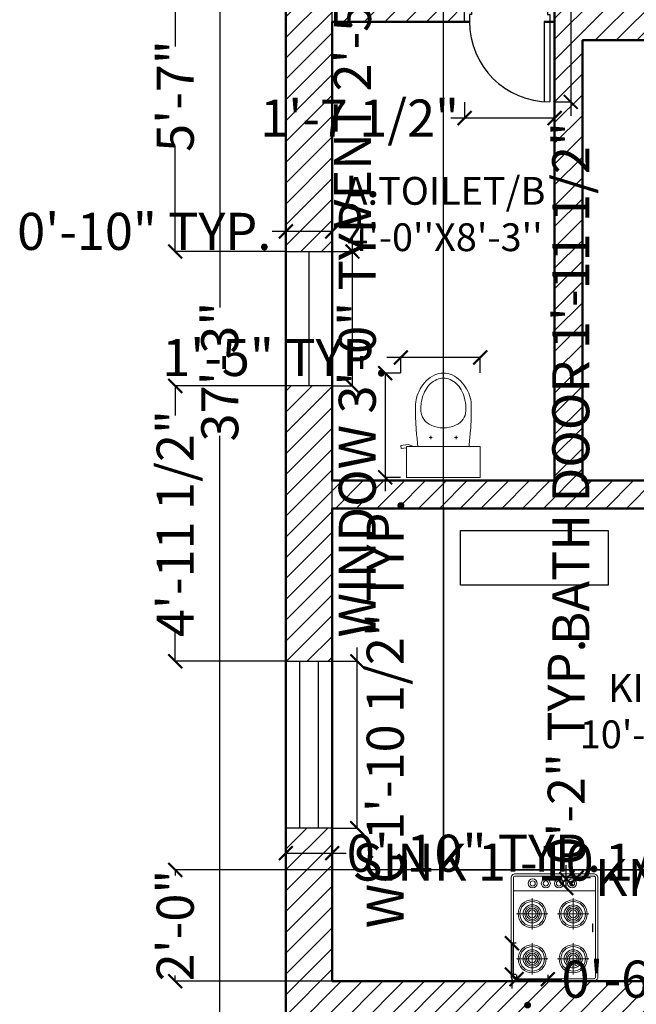
# Model space of a CAD drawing. Units: inches. Extents: x 1945 to 2401, y 1770 to 2289.
# Tile 2 of 5: x 1945 to 2078, y 1893 to 2105. Entities that reach past the tile are written whole.
import ezdxf

# ---------------------------------------------------------------- set-up
doc = ezdxf.new("R2010")
doc.units = ezdxf.units.IN
for name, color, linetype, lineweight in [('A-ANNO-DIMS', 2, 'Continuous', 18), ('A-AREA-IDEN', 7, 'Continuous', 25), ('A-EQPM', 9, 'Continuous', 18), ('A-FLOR-FIXT', 9, 'Continuous', 18), ('A-WALL-PATT', 8, 'Continuous', 13), ('Doors', 150, 'Continuous', 25), ('kitchen', 122, 'Continuous', 25), ('Walls', 7, 'Continuous', 50), ('Windows', 32, 'Continuous', 25)]:
    doc.layers.add(name, color=color, linetype=linetype, lineweight=lineweight)
doc.styles.get("Standard").update_dxf_attribs({"font": 'arial.ttf'})
doc.dimstyles.get("Standard").update_dxf_attribs({"dimtxt": 8, "dimasz": 3, "dimexe": 0.18, "dimexo": 0.0625, "dimgap": 0.09, "dimtad": 0, "dimdec": 1, "dimzin": 0, "dimdsep": 46, "dimlunit": 4, "dimtxsty": 'Standard', "dimblk": 'ARCHTICK', "dimcen": 0.09, "dimadec": 0, "dimazin": 0, "dimtfac": 1, "dimtdec": 1, "dimtofl": 0, "dimtmove": 0, "dimatfit": 3, "dimfxl": 1, "dimtolj": 1, "dimtzin": 0, "dimarcsym": 0})

# ---------------------------------------------------------------- blocks, each defined once
blk = doc.blocks.new('toilet-1')
at = {"color": 0, "linetype": 'ByBlock'}
for p, q in [((-0.23, -0.02), (-0.23, -0.2116)), ((0.23, -0.02), (-0.23, -0.02)), ((0.23, -0.02), (0.23, -0.2116)), ((-0.23, -0.2116), (0.23, -0.2116)), ((0.1917, -0.2144), (0.2206, -0.225)), ((0.2206, -0.225), (0.266, -0.2187)), ((0.2633, -0.1997), (0.23, -0.2044)), ((0.266, -0.2187), (0.2633, -0.1997)), ((-0.0889, -0.2683), (-0.0697, -0.2683)), ((-0.0793, -0.2587), (-0.0793, -0.2778)), ((0.0889, -0.2683), (0.0698, -0.2683)), ((0.0794, -0.2587), (0.0794, -0.2778)), ((0, -0.6382), (0, -0.6382))]:
    blk.add_line(p, q, dxfattribs=at)
for centre, radius, start, end in [((3.5272, -0.6239), 3.7093, 173.69251, 175.15926), ((-3.527, -0.624), 3.7093, 4.84131, 6.31706), ((1.7368, -0.4519), 1.9109, 175.76982, 180.37578), ((-0.0312, -0.4465), 0.1114, 113.89968, 145.1485), ((0, -0.5169), 0.1884, 66.09393, 113.90607), ((0.0312, -0.4465), 0.1114, 34.8515, 66.10032), ((-1.7366, -0.4519), 1.9109, 359.62422, 4.23018), ((-0.0408, -0.4398), 0.0996, 145.14967, 175.88096), ((0.0409, -0.4398), 0.0996, 4.11904, 34.85033), ((0.0353, -0.463), 0.2093, 180.37466, 194.33753), ((0.0981, -0.4497), 0.2389, 175.88621, 195.59308), ((-0.098, -0.4497), 0.2389, 344.40692, 4.11379), ((-0.0351, -0.463), 0.2093, 345.6614, 359.62427), ((0.055, -0.458), 0.2297, 194.33532, 209.62204), ((0.0961, -0.4503), 0.2369, 195.59686, 209.37705), ((-0.096, -0.4503), 0.2369, 330.62295, 344.40314), ((-0.0548, -0.458), 0.2297, 330.37879, 345.66551), ((0.0647, -0.4524), 0.2409, 209.62726, 224.54888), ((0.0232, -0.4913), 0.1532, 209.38715, 226.54376), ((0.0152, -0.4997), 0.1416, 226.55015, 246.55272), ((-0.0151, -0.4997), 0.1416, 293.44728, 313.44985), ((-0.0231, -0.4913), 0.1532, 313.45624, 330.61285), ((-0.0645, -0.4524), 0.2409, 315.45042, 330.37204), ((0.0178, -0.4986), 0.1751, 224.55199, 245.714), ((0.0004, -0.538), 0.132, 245.58449, 269.87817), ((0, -0.5347), 0.1034, 246.54933, 270.0042), ((0, -0.5347), 0.1034, 269.9958, 293.45067), ((-0.0002, -0.538), 0.132, 270.12162, 294.4153), ((-0.0176, -0.4986), 0.1751, 294.28649, 315.4485)]:
    blk.add_arc(centre, radius, start, end, dxfattribs=at)
blk = doc.blocks.new('AP0B01')
blk.add_line((75, 100), (75, 678.7))
blk.add_lwpolyline([(35, 100), (35, 680, -0.449922)], format="xyb")
for points in [[(0, 100), (0, -100), (35, -100), (35, -50), (50, -50), (50, 50), (35, 50), (35, 100)], [(650, 100), (650, -100), (615, -100), (615, -50), (600, -50), (600, 50), (615, 50), (615, 100)]]:
    blk.add_lwpolyline(points, close=True)
blk.add_lwpolyline([(35, 100), (75, 100)])
blk.add_arc((35, 100), 580, 0, 90)
blk = doc.blocks.new('_ArchTick')
at = {"color": 0, "linetype": 'ByBlock', "const_width": 0.15}
blk.add_lwpolyline([(-0.5, -0.5), (0.5, 0.5)], dxfattribs=at)
blk = doc.blocks.new('*D20')
at = {"layer": 'A-ANNO-DIMS', "color": 0, "lineweight": -2, "transparency": 16777216}
for p, q in [((2002.78, 2253.04), (1988.38, 2253.04)), ((1988.56, 2253.04), (1988.56, 2043.37)), ((1988.56, 1806.04), (1988.56, 2015.71)), ((2002.78, 1806.04), (1988.38, 1806.04))]:
    blk.add_line(p, q, dxfattribs=at)
at = {"layer": 'Defpoints', "color": 0, "transparency": 16777216}
for p in [(2002.84, 2253.04), (1988.56, 1806.04), (2002.84, 1806.04)]:
    blk.add_point(p, dxfattribs=at)
at = {"layer": 'A-ANNO-DIMS', "color": 0, "lineweight": -2, "transparency": 16777216, "xscale": 3, "yscale": 3, "zscale": 3}
for p, rotation in [((1988.56, 2253.04), 90), ((1988.56, 1806.04), 270)]:
    blk.add_blockref('_ArchTick', p, dxfattribs=dict(at, rotation=rotation))
at = {"layer": 'A-ANNO-DIMS', "color": 0, "transparency": 16777216, "insert": (1988.56, 2029.54), "char_height": 8, "attachment_point": 5, "rotation": 90}
blk.add_mtext('\\A1;37\'-3"', dxfattribs=at)
blk = doc.blocks.new('WIN-36IN')
for p, q in [((3, 0), (3, 36)), ((7, 0), (7, 36))]:
    blk.add_line(p, q)
blk.add_lwpolyline([(0, 0), (0, 36), (10, 36), (10, 0)], close=True)
blk = doc.blocks.new('VENT-WIN-29IN')
blk.add_line((0, 5), (29, 5))
blk.add_lwpolyline([(0, 10), (29, 10), (29, 0), (0, 0)], close=True)
blk = doc.blocks.new('COOKTOP-BURNER')
for p, q in [((3.36, 0), (3.36, 6.73)), ((0, 3.36), (6.73, 3.36))]:
    blk.add_line(p, q)
for radius in [3.01, 2.66, 1.95, 1.59, 1.24, 0.85]:
    blk.add_circle((3.36, 3.36), radius)
blk = doc.blocks.new('COOKTOP-KNOB')
for radius in [0.974, 0.554]:
    blk.add_circle((0.97, 0.97), radius)
blk = doc.blocks.new('*D29')
at = {"layer": 'A-ANNO-DIMS', "color": 0, "lineweight": -2, "transparency": 16777216}
for p, q in [((2052.57, 1906.21), (2051.45, 1906.21)), ((2051.63, 1906.21), (2051.63, 1899.48)), ((2052.57, 1899.48), (2051.45, 1899.48)), ((2051.63, 1899.48), (2051.63, 1896.48))]:
    blk.add_line(p, q, dxfattribs=at)
at = {"layer": 'Defpoints', "color": 0, "transparency": 16777216}
for p in [(2052.64, 1906.21), (2051.63, 1899.48), (2052.64, 1899.48)]:
    blk.add_point(p, dxfattribs=at)
at = {"layer": 'A-ANNO-DIMS', "color": 0, "lineweight": -2, "transparency": 16777216, "xscale": 3, "yscale": 3, "zscale": 3}
for p, rotation in [((2051.63, 1906.21), 90), ((2051.63, 1899.48), 270)]:
    blk.add_blockref('_ArchTick', p, dxfattribs=dict(at, rotation=rotation))
at = {"layer": 'A-ANNO-DIMS', "color": 0, "transparency": 16777216, "insert": (2051.63, 1837.71), "char_height": 8, "attachment_point": 5, "rotation": 90}
blk.add_mtext('\\A1;BURNER 0\'-6 1/2" TYP.', dxfattribs=at)
blk = doc.blocks.new('*D30')
at = {"layer": 'A-ANNO-DIMS', "color": 0, "lineweight": -2, "transparency": 16777216}
for p, q in [((2052.64, 1899.41), (2052.64, 1898.29)), ((2059.37, 1899.41), (2059.37, 1898.29)), ((2052.64, 1898.47), (2059.37, 1898.47)), ((2059.37, 1898.47), (2062.37, 1898.47))]:
    blk.add_line(p, q, dxfattribs=at)
at = {"layer": 'Defpoints', "color": 0, "transparency": 16777216}
for p in [(2052.64, 1899.48), (2059.37, 1899.48), (2059.37, 1898.47)]:
    blk.add_point(p, dxfattribs=at)
at = {"layer": 'A-ANNO-DIMS', "color": 0, "lineweight": -2, "transparency": 16777216, "xscale": 3, "yscale": 3, "zscale": 3, "rotation": 180}
blk.add_blockref('_ArchTick', (2052.64, 1898.47), dxfattribs=at)
at = {"layer": 'A-ANNO-DIMS', "color": 0, "lineweight": -2, "transparency": 16777216, "xscale": 3, "yscale": 3, "zscale": 3}
blk.add_blockref('_ArchTick', (2059.37, 1898.47), dxfattribs=at)
at = {"layer": 'A-ANNO-DIMS', "color": 0, "transparency": 16777216, "insert": (2096.16, 1898.47), "char_height": 8, "attachment_point": 5}
blk.add_mtext('\\A1;0\'-6 1/2" TYP.', dxfattribs=at)
blk = doc.blocks.new('*D31')
at = {"layer": 'A-ANNO-DIMS', "color": 0, "lineweight": -2, "transparency": 16777216}
for p, q in [((2063.65, 1920.15), (2063.65, 1920.56)), ((2063.65, 1920.38), (2065.6, 1920.38)), ((2065.6, 1920.15), (2065.6, 1920.56)), ((2065.6, 1920.38), (2068.6, 1920.38))]:
    blk.add_line(p, q, dxfattribs=at)
at = {"layer": 'Defpoints', "color": 0, "transparency": 16777216}
for p in [(2065.6, 1920.38), (2063.65, 1920.08), (2065.6, 1920.08)]:
    blk.add_point(p, dxfattribs=at)
at = {"layer": 'A-ANNO-DIMS', "color": 0, "lineweight": -2, "transparency": 16777216, "xscale": 3, "yscale": 3, "zscale": 3, "rotation": 180}
blk.add_blockref('_ArchTick', (2063.65, 1920.38), dxfattribs=at)
at = {"layer": 'A-ANNO-DIMS', "color": 0, "lineweight": -2, "transparency": 16777216, "xscale": 3, "yscale": 3, "zscale": 3}
blk.add_blockref('_ArchTick', (2065.6, 1920.38), dxfattribs=at)
at = {"layer": 'A-ANNO-DIMS', "color": 0, "transparency": 16777216, "insert": (2110.28, 1920.38), "char_height": 8, "attachment_point": 5}
blk.add_mtext('\\A1;KNOB 0\'-2" TYP.', dxfattribs=at)
blk = doc.blocks.new('*D32')
at = {"layer": 'A-ANNO-DIMS', "color": 0, "lineweight": -2, "transparency": 16777216}
for p, q in [((2063.36, 1920.08), (2063.36, 1923.08)), ((2063.59, 1920.08), (2063.18, 1920.08)), ((2063.36, 1918.14), (2063.36, 1920.08)), ((2063.59, 1918.14), (2063.18, 1918.14))]:
    blk.add_line(p, q, dxfattribs=at)
at = {"layer": 'Defpoints', "color": 0, "transparency": 16777216}
for p in [(2063.36, 1920.08), (2063.65, 1920.08), (2063.65, 1918.14)]:
    blk.add_point(p, dxfattribs=at)
at = {"layer": 'A-ANNO-DIMS', "color": 0, "lineweight": -2, "transparency": 16777216, "xscale": 3, "yscale": 3, "zscale": 3}
for p, rotation in [((2063.36, 1920.08), 90), ((2063.36, 1918.14), 270)]:
    blk.add_blockref('_ArchTick', p, dxfattribs=dict(at, rotation=rotation))
at = {"layer": 'A-ANNO-DIMS', "color": 0, "transparency": 16777216, "insert": (2063.36, 1947.56), "char_height": 8, "attachment_point": 5, "rotation": 90}
blk.add_mtext('\\A1;0\'-2" TYP.', dxfattribs=at)
blk = doc.blocks.new('*D41')
at = {"layer": 'A-ANNO-DIMS', "color": 0, "lineweight": -2, "transparency": 16777216}
for p, q in [((2027.58, 2029.22), (2024.09, 2029.22)), ((2024.27, 2029.22), (2024.27, 2006.73)), ((2027.58, 2006.73), (2024.09, 2006.73)), ((2024.27, 2006.73), (2024.27, 2003.73))]:
    blk.add_line(p, q, dxfattribs=at)
at = {"layer": 'Defpoints', "color": 0, "transparency": 16777216}
for p in [(2027.64, 2029.22), (2024.27, 2006.73), (2027.64, 2006.73)]:
    blk.add_point(p, dxfattribs=at)
at = {"layer": 'A-ANNO-DIMS', "color": 0, "lineweight": -2, "transparency": 16777216, "xscale": 3, "yscale": 3, "zscale": 3}
for p, rotation in [((2024.27, 2029.22), 90), ((2024.27, 2006.73), 270)]:
    blk.add_blockref('_ArchTick', p, dxfattribs=dict(at, rotation=rotation))
at = {"layer": 'A-ANNO-DIMS', "color": 0, "transparency": 16777216, "insert": (2024.27, 1955.81), "char_height": 8, "attachment_point": 5, "rotation": 90}
blk.add_mtext('\\A1;WC 1\'-10 1/2" TYP.', dxfattribs=at)
blk = doc.blocks.new('*D42')
at = {"layer": 'A-ANNO-DIMS', "color": 0, "lineweight": -2, "transparency": 16777216}
for p, q in [((2027.64, 2032.59), (2024.64, 2032.59)), ((2027.64, 2029.28), (2027.64, 2032.77)), ((2044.8, 2032.59), (2027.64, 2032.59)), ((2044.8, 2029.28), (2044.8, 2032.77))]:
    blk.add_line(p, q, dxfattribs=at)
at = {"layer": 'Defpoints', "color": 0, "transparency": 16777216}
for p in [(2027.64, 2032.59), (2027.64, 2029.22), (2044.8, 2029.22)]:
    blk.add_point(p, dxfattribs=at)
at = {"layer": 'A-ANNO-DIMS', "color": 0, "lineweight": -2, "transparency": 16777216, "xscale": 3, "yscale": 3, "zscale": 3, "rotation": 180}
blk.add_blockref('_ArchTick', (2027.64, 2032.59), dxfattribs=at)
at = {"layer": 'A-ANNO-DIMS', "color": 0, "lineweight": -2, "transparency": 16777216, "xscale": 3, "yscale": 3, "zscale": 3}
blk.add_blockref('_ArchTick', (2044.8, 2032.59), dxfattribs=at)
at = {"layer": 'A-ANNO-DIMS', "color": 0, "transparency": 16777216, "insert": (2000.54, 2032.59), "char_height": 8, "attachment_point": 5}
blk.add_mtext('\\A1;1\'-5" TYP.', dxfattribs=at)
blk = doc.blocks.new('*D43')
at = {"layer": 'A-ANNO-DIMS', "color": 0, "lineweight": -2, "transparency": 16777216}
for p, q in [((2060.9, 2111.04), (2064.52, 2111.04)), ((2064.34, 2111.04), (2064.34, 2087.72)), ((2060.9, 2087.72), (2064.52, 2087.72)), ((2064.34, 2087.72), (2064.34, 2084.72))]:
    blk.add_line(p, q, dxfattribs=at)
at = {"layer": 'Defpoints', "color": 0, "transparency": 16777216}
for p in [(2060.84, 2111.04), (2060.84, 2087.72), (2064.34, 2087.72)]:
    blk.add_point(p, dxfattribs=at)
at = {"layer": 'A-ANNO-DIMS', "color": 0, "lineweight": -2, "transparency": 16777216, "xscale": 3, "yscale": 3, "zscale": 3}
for p, rotation in [((2064.34, 2111.04), 90), ((2064.34, 2087.72), 270)]:
    blk.add_blockref('_ArchTick', p, dxfattribs=dict(at, rotation=rotation))
at = {"layer": 'A-ANNO-DIMS', "color": 0, "transparency": 16777216, "insert": (2064.34, 2026.98), "char_height": 8, "attachment_point": 5, "rotation": 90}
blk.add_mtext('\\A1;BATH DOOR 1\'-11 1/2"', dxfattribs=at)
blk = doc.blocks.new('*D44')
at = {"layer": 'A-ANNO-DIMS', "color": 0, "lineweight": -2, "transparency": 16777216}
for p, q in [((2041.41, 2087.66), (2041.41, 2084.05)), ((2060.84, 2087.66), (2060.84, 2084.05)), ((2041.41, 2084.23), (2038.41, 2084.23)), ((2060.84, 2084.23), (2041.41, 2084.23))]:
    blk.add_line(p, q, dxfattribs=at)
at = {"layer": 'Defpoints', "color": 0, "transparency": 16777216}
for p in [(2041.41, 2087.72), (2060.84, 2087.72), (2041.41, 2084.23)]:
    blk.add_point(p, dxfattribs=at)
at = {"layer": 'A-ANNO-DIMS', "color": 0, "lineweight": -2, "transparency": 16777216, "xscale": 3, "yscale": 3, "zscale": 3, "rotation": 180}
blk.add_blockref('_ArchTick', (2041.41, 2084.23), dxfattribs=at)
at = {"layer": 'A-ANNO-DIMS', "color": 0, "lineweight": -2, "transparency": 16777216, "xscale": 3, "yscale": 3, "zscale": 3}
blk.add_blockref('_ArchTick', (2060.84, 2084.23), dxfattribs=at)
at = {"layer": 'A-ANNO-DIMS', "color": 0, "transparency": 16777216, "insert": (2018.75, 2084.23), "char_height": 8, "attachment_point": 5}
blk.add_mtext('\\A1;1\'-7 1/2"', dxfattribs=at)
blk = doc.blocks.new('*D49')
at = {"layer": 'A-ANNO-DIMS', "color": 0, "lineweight": -2, "transparency": 16777216}
for p, q in [((2018.24, 1967.04), (2018.24, 1970.04)), ((2012.9, 1967.04), (2018.42, 1967.04)), ((2018.24, 1931.04), (2018.24, 1967.04)), ((2012.9, 1931.04), (2018.42, 1931.04))]:
    blk.add_line(p, q, dxfattribs=at)
at = {"layer": 'Defpoints', "color": 0, "transparency": 16777216}
for p in [(2012.84, 1967.04), (2018.24, 1967.04), (2012.84, 1931.04)]:
    blk.add_point(p, dxfattribs=at)
at = {"layer": 'A-ANNO-DIMS', "color": 0, "lineweight": -2, "transparency": 16777216, "xscale": 3, "yscale": 3, "zscale": 3}
for p, rotation in [((2018.24, 1967.04), 90), ((2018.24, 1931.04), 270)]:
    blk.add_blockref('_ArchTick', p, dxfattribs=dict(at, rotation=rotation))
at = {"layer": 'A-ANNO-DIMS', "color": 0, "transparency": 16777216, "insert": (2018.24, 2020.75), "char_height": 8, "attachment_point": 5, "rotation": 90}
blk.add_mtext('\\A1;WINDOW 3\'-0" TYP.', dxfattribs=at)
blk = doc.blocks.new('*D50')
at = {"layer": 'A-ANNO-DIMS', "color": 0, "lineweight": -2, "transparency": 16777216}
for p, q in [((2002.84, 1930.98), (2002.84, 1925.46)), ((2012.84, 1930.98), (2012.84, 1925.46)), ((2002.84, 1925.64), (2012.84, 1925.64)), ((2012.84, 1925.64), (2015.84, 1925.64))]:
    blk.add_line(p, q, dxfattribs=at)
at = {"layer": 'Defpoints', "color": 0, "transparency": 16777216}
for p in [(2002.84, 1931.04), (2012.84, 1931.04), (2012.84, 1925.64)]:
    blk.add_point(p, dxfattribs=at)
at = {"layer": 'A-ANNO-DIMS', "color": 0, "lineweight": -2, "transparency": 16777216, "xscale": 3, "yscale": 3, "zscale": 3, "rotation": 180}
blk.add_blockref('_ArchTick', (2002.84, 1925.64), dxfattribs=at)
at = {"layer": 'A-ANNO-DIMS', "color": 0, "lineweight": -2, "transparency": 16777216, "xscale": 3, "yscale": 3, "zscale": 3}
blk.add_blockref('_ArchTick', (2012.84, 1925.64), dxfattribs=at)
at = {"layer": 'A-ANNO-DIMS', "color": 0, "transparency": 16777216, "insert": (2043.42, 1925.64), "char_height": 8, "attachment_point": 5}
blk.add_mtext('\\A1;0\'-10" TYP.', dxfattribs=at)
blk = doc.blocks.new('*D51')
at = {"layer": 'A-ANNO-DIMS', "color": 0, "lineweight": -2, "transparency": 16777216}
for p, q in [((2017.19, 2055.45), (2017.19, 2058.45)), ((2012.9, 2055.45), (2017.37, 2055.45)), ((2017.19, 2026.45), (2017.19, 2055.45)), ((2012.9, 2026.45), (2017.37, 2026.45))]:
    blk.add_line(p, q, dxfattribs=at)
at = {"layer": 'Defpoints', "color": 0, "transparency": 16777216}
for p in [(2012.84, 2055.45), (2017.19, 2055.45), (2012.84, 2026.45)]:
    blk.add_point(p, dxfattribs=at)
at = {"layer": 'A-ANNO-DIMS', "color": 0, "lineweight": -2, "transparency": 16777216, "xscale": 3, "yscale": 3, "zscale": 3}
for p, rotation in [((2017.19, 2055.45), 90), ((2017.19, 2026.45), 270)]:
    blk.add_blockref('_ArchTick', p, dxfattribs=dict(at, rotation=rotation))
at = {"layer": 'A-ANNO-DIMS', "color": 0, "transparency": 16777216, "insert": (2017.19, 2099.59), "char_height": 8, "attachment_point": 5, "rotation": 90}
blk.add_mtext('\\A1;VENT 2\'-5" TYP.', dxfattribs=at)
blk = doc.blocks.new('*D52')
at = {"layer": 'A-ANNO-DIMS', "color": 0, "lineweight": -2, "transparency": 16777216}
for p, q in [((2002.84, 2059.8), (1999.84, 2059.8)), ((2002.84, 2055.51), (2002.84, 2059.98)), ((2012.84, 2059.8), (2002.84, 2059.8)), ((2012.84, 2055.51), (2012.84, 2059.98))]:
    blk.add_line(p, q, dxfattribs=at)
at = {"layer": 'Defpoints', "color": 0, "transparency": 16777216}
for p in [(2002.84, 2059.8), (2002.84, 2055.45), (2012.84, 2055.45)]:
    blk.add_point(p, dxfattribs=at)
at = {"layer": 'A-ANNO-DIMS', "color": 0, "lineweight": -2, "transparency": 16777216, "xscale": 3, "yscale": 3, "zscale": 3}
for p, rotation in [((2002.84, 2059.8), 180.0000000000025), ((2012.84, 2059.8), 2.558e-12)]:
    blk.add_blockref('_ArchTick', p, dxfattribs=dict(at, rotation=rotation))
at = {"layer": 'A-ANNO-DIMS', "color": 0, "transparency": 16777216, "insert": (1972.26, 2059.8), "char_height": 8, "attachment_point": 5}
blk.add_mtext('\\A1;0\'-10" TYP.', dxfattribs=at)
blk = doc.blocks.new('*D57')
at = {"layer": 'A-ANNO-DIMS', "color": 0, "lineweight": -2, "transparency": 16777216}
for p, q in [((2095.97, 1923.73), (2092.97, 1923.73)), ((2095.97, 1920.44), (2095.97, 1923.91)), ((2118.35, 1923.73), (2095.97, 1923.73)), ((2118.35, 1920.44), (2118.35, 1923.91))]:
    blk.add_line(p, q, dxfattribs=at)
at = {"layer": 'Defpoints', "color": 0, "transparency": 16777216}
for p in [(2095.97, 1923.73), (2095.97, 1920.38), (2118.35, 1920.38)]:
    blk.add_point(p, dxfattribs=at)
at = {"layer": 'A-ANNO-DIMS', "color": 0, "lineweight": -2, "transparency": 16777216, "xscale": 3, "yscale": 3, "zscale": 3, "rotation": 180}
blk.add_blockref('_ArchTick', (2095.97, 1923.73), dxfattribs=at)
at = {"layer": 'A-ANNO-DIMS', "color": 0, "lineweight": -2, "transparency": 16777216, "xscale": 3, "yscale": 3, "zscale": 3}
blk.add_blockref('_ArchTick', (2118.35, 1923.73), dxfattribs=at)
at = {"layer": 'A-ANNO-DIMS', "color": 0, "transparency": 16777216, "insert": (2055.24, 1923.73), "char_height": 8, "attachment_point": 5}
blk.add_mtext('\\A1;SINK 1\'-10 1/2"', dxfattribs=at)
blk = doc.blocks.new('*D63')
at = {"layer": 'A-ANNO-DIMS', "color": 0, "lineweight": -2, "transparency": 16777216}
for p, q in [((2002.78, 2122.54), (1978.76, 2122.54)), ((1978.94, 2122.54), (1978.94, 2099.72)), ((1978.94, 2055.45), (1978.94, 2078.27)), ((2002.78, 2055.45), (1978.76, 2055.45))]:
    blk.add_line(p, q, dxfattribs=at)
at = {"layer": 'Defpoints', "color": 0, "transparency": 16777216}
for p in [(2002.84, 2122.54), (1978.94, 2055.45), (2002.84, 2055.45)]:
    blk.add_point(p, dxfattribs=at)
at = {"layer": 'A-ANNO-DIMS', "color": 0, "lineweight": -2, "transparency": 16777216, "xscale": 3, "yscale": 3, "zscale": 3}
for p, rotation in [((1978.94, 2122.54), 90), ((1978.94, 2055.45), 270)]:
    blk.add_blockref('_ArchTick', p, dxfattribs=dict(at, rotation=rotation))
at = {"layer": 'A-ANNO-DIMS', "color": 0, "transparency": 16777216, "insert": (1978.94, 2089), "char_height": 8, "attachment_point": 5, "rotation": 90}
blk.add_mtext('\\A1;5\'-7"', dxfattribs=at)
blk = doc.blocks.new('*D64')
at = {"layer": 'A-ANNO-DIMS', "color": 0, "lineweight": -2, "transparency": 16777216}
for p, q in [((2002.78, 2026.45), (1978.76, 2026.45)), ((1978.94, 2026.45), (1978.94, 2020.06)), ((1978.94, 1967.04), (1978.94, 1973.43)), ((2002.78, 1967.04), (1978.76, 1967.04))]:
    blk.add_line(p, q, dxfattribs=at)
at = {"layer": 'Defpoints', "color": 0, "transparency": 16777216}
for p in [(2002.84, 2026.45), (1978.94, 1967.04), (2002.84, 1967.04)]:
    blk.add_point(p, dxfattribs=at)
at = {"layer": 'A-ANNO-DIMS', "color": 0, "lineweight": -2, "transparency": 16777216, "xscale": 3, "yscale": 3, "zscale": 3}
for p, rotation in [((1978.94, 2026.45), 90), ((1978.94, 1967.04), 270)]:
    blk.add_blockref('_ArchTick', p, dxfattribs=dict(at, rotation=rotation))
at = {"layer": 'A-ANNO-DIMS', "color": 0, "transparency": 16777216, "insert": (1978.94, 1996.75), "char_height": 8, "attachment_point": 5, "rotation": 90}
blk.add_mtext('\\A1;4\'-11 1/2"', dxfattribs=at)
blk = doc.blocks.new('*D67')
at = {"layer": 'A-ANNO-DIMS', "color": 0, "lineweight": -2, "transparency": 16777216}
for p, q in [((2012.84, 1931.1), (2012.84, 2277.12)), ((2012.84, 2276.94), (2014.05, 2276.94)), ((2036.84, 2276.94), (2035.63, 2276.94)), ((2036.84, 1922.1), (2036.84, 2277.12))]:
    blk.add_line(p, q, dxfattribs=at)
at = {"layer": 'Defpoints', "color": 0, "transparency": 16777216}
for p in [(2036.84, 2276.94), (2012.84, 1931.04), (2036.84, 1922.04)]:
    blk.add_point(p, dxfattribs=at)
at = {"layer": 'A-ANNO-DIMS', "color": 0, "lineweight": -2, "transparency": 16777216, "xscale": 3, "yscale": 3, "zscale": 3, "rotation": 180}
blk.add_blockref('_ArchTick', (2012.84, 2276.94), dxfattribs=at)
at = {"layer": 'A-ANNO-DIMS', "color": 0, "lineweight": -2, "transparency": 16777216, "xscale": 3, "yscale": 3, "zscale": 3}
blk.add_blockref('_ArchTick', (2036.84, 2276.94), dxfattribs=at)
at = {"layer": 'A-ANNO-DIMS', "color": 0, "transparency": 16777216, "insert": (2024.84, 2276.94), "char_height": 8, "attachment_point": 5}
blk.add_mtext('\\A1;2\'-0"', dxfattribs=at)
blk = doc.blocks.new('*D68')
at = {"layer": 'A-ANNO-DIMS', "color": 0, "lineweight": -2, "transparency": 16777216}
for p, q in [((2132.78, 1922.04), (1978.76, 1922.04)), ((1978.94, 1922.04), (1978.94, 1920.83)), ((1978.94, 1898.04), (1978.94, 1899.25)), ((2132.78, 1898.04), (1978.76, 1898.04))]:
    blk.add_line(p, q, dxfattribs=at)
at = {"layer": 'Defpoints', "color": 0, "transparency": 16777216}
for p in [(1978.94, 1922.04), (2132.84, 1922.04), (2132.84, 1898.04)]:
    blk.add_point(p, dxfattribs=at)
at = {"layer": 'A-ANNO-DIMS', "color": 0, "lineweight": -2, "transparency": 16777216, "xscale": 3, "yscale": 3, "zscale": 3}
for p, rotation in [((1978.94, 1922.04), 90), ((1978.94, 1898.04), 270)]:
    blk.add_blockref('_ArchTick', p, dxfattribs=dict(at, rotation=rotation))
at = {"layer": 'A-ANNO-DIMS', "color": 0, "transparency": 16777216, "insert": (1978.94, 1910.04), "char_height": 8, "attachment_point": 5, "rotation": 90}
blk.add_mtext('\\A1;2\'-0"', dxfattribs=at)

msp = doc.modelspace()

# ---------------------------------------------------------------- hatches: boundary and pattern name
at = {"layer": 'A-WALL-PATT', "transparency": 33554585}
h = msp.add_hatch(dxfattribs=at)
h.set_pattern_fill('ANSI31', color=256)
h.paths.add_polyline_path([(2151.34, 2253.04), (2002.84, 2253.04), (2002.84, 2158.54), (2012.84, 2158.54), (2012.84, 2243.04), (2132.84, 2243.04), (2132.88, 2160.39), (2142.84, 2160.39), (2142.84, 2165.04), (2192.84, 2165.04), (2192.84, 2160.39), (2202.84, 2160.39), (2202.84, 2175.04), (2192.84, 2175.04), (2192.84, 2171.04), (2138.84, 2171.04), (2138.84, 2243.04), (2151.34, 2243.04)])
h.paths.add_polyline_path([(2332.84, 2253.04), (2180.34, 2253.04), (2180.34, 2243.04), (2192.84, 2243.04), (2192.84, 2207.47), (2202.84, 2207.47), (2202.84, 2243.04), (2322.84, 2243.04), (2322.84, 2175.57), (2332.84, 2175.57)])
h.paths.add_polyline_path([(2012.84, 2105.04), (2041.41, 2105.04), (2041.41, 2111.04), (2012.84, 2111.04), (2012.84, 2122.54), (2002.84, 2122.54), (2002.84, 2055.45), (2012.84, 2055.45)])
h.paths.add_polyline_path([(2332.84, 2115.57), (2322.84, 2115.57), (2322.84, 2111.04), (2202.84, 2111.04), (2202.84, 2118.04), (2192.84, 2118.04), (2192.84, 2111.04), (2181.84, 2111.04), (2181.84, 2101.04), (2322.84, 2101.04), (2322.84, 2041.04), (2332.84, 2041.04)])
h = msp.add_hatch(dxfattribs=at)
h.set_pattern_fill('ANSI31', color=256)
h.paths.add_polyline_path([(2142.84, 2006.04), (2132.84, 2006.04), (2132.84, 1898.04), (2012.84, 1898.04), (2012.84, 1888.04), (2142.84, 1888.04), (2142.84, 1911.04), (2179.42, 1911.04), (2179.42, 1921.04), (2142.84, 1921.04)])
h.paths.add_polyline_path([(2269.5, 1921.04), (2239.42, 1921.04), (2239.42, 1911.04), (2269.5, 1911.04)])
h.paths.add_polyline_path([(2332.84, 1981.04), (2322.84, 1981.04), (2322.84, 1921.04), (2311.84, 1921.04), (2311.84, 1911.04), (2322.84, 1911.04), (2322.84, 1817.97), (2332.84, 1817.97)])
h.paths.add_polyline_path([(2012.84, 1931.04), (2002.84, 1931.04), (2002.84, 1806.04), (2142.84, 1806.04), (2142.84, 1816.04), (2012.84, 1816.04)])
h.paths.add_polyline_path([(2012.84, 2000.04), (2082.92, 2000.04), (2082.92, 2006.04), (2066.84, 2006.04), (2066.84, 2101.04), (2142.84, 2101.04), (2153.84, 2101.04), (2153.84, 2111.04), (2142.84, 2111.04), (2142.84, 2118.04), (2132.84, 2118.04), (2132.84, 2111.04), (2060.84, 2111.04), (2060.84, 2006.04), (2012.84, 2006.04), (2012.84, 2026.45), (2002.84, 2026.45), (2002.84, 1967.04), (2012.84, 1967.04)])

# ---------------------------------------------------------------- linework, layer by layer
at = {"layer": 'A-EQPM'}
msp.add_line((2069.67, 1917.52), (2051.96, 1917.52), dxfattribs=at)
for points in [[(2051.47, 1898.93), (2051.47, 1920.32, -0.414214), (2052.35, 1921.2), (2069.28, 1921.2, -0.414214), (2070.17, 1920.32), (2070.17, 1898.93, -0.414214), (2069.28, 1898.04), (2052.35, 1898.04, -0.414214)], [(2051.96, 1898.93), (2051.96, 1920.32, -0.414214), (2052.35, 1920.7), (2069.28, 1920.7, -0.414214), (2069.67, 1920.32), (2069.67, 1898.93, -0.414214), (2069.28, 1898.54), (2052.35, 1898.54, -0.414214)]]:
    msp.add_lwpolyline(points, format="xyb", close=True, dxfattribs=at)
msp.add_lwpolyline([(2069.1, 1910.43), (2069.1, 1908.66), (2069.03, 1908.66), (2069.03, 1910.43)], close=True, dxfattribs=at)
at = {"layer": 'kitchen'}
for p, q in [((2036.84, 2000.04), (2036.84, 1922.04)), ((2036.84, 1922.04), (2132.84, 1922.04))]:
    msp.add_line(p, q, dxfattribs=at)
msp.add_lwpolyline([(2040.5, 1995.26), (2072.4, 1995.26), (2072.4, 1983.44), (2040.5, 1983.44)], close=True, dxfattribs=at)
at = {"layer": 'Walls'}
for p, q in [((2002.84, 2253.04), (2002.84, 1806.04)), ((2060.84, 2111.04), (2060.84, 2006.04)), ((2012.84, 2105.04), (2042.46, 2105.04)), ((2012.84, 2105.04), (2012.84, 2006.04)), ((2058.6, 2105.04), (2060.84, 2105.04)), ((2066.84, 2101.04), (2066.84, 2006.04)), ((2066.84, 2101.04), (2142.84, 2101.04)), ((2012.84, 2006.04), (2060.84, 2006.04)), ((2066.84, 2006.04), (2082.92, 2006.04)), ((2012.84, 2000.04), (2082.92, 2000.04)), ((2012.84, 2000.04), (2012.84, 1898.04)), ((2012.84, 1898.04), (2132.84, 1898.04))]:
    msp.add_line(p, q, dxfattribs=at)

# ---------------------------------------------------------------- block references
at = {"layer": 'A-EQPM'}
for name, p in [('COOKTOP-KNOB', (2055.15, 1918.14)), ('COOKTOP-KNOB', (2057.98, 1918.14)), ('COOKTOP-KNOB', (2060.82, 1918.14)), ('COOKTOP-KNOB', (2063.65, 1918.14)), ('COOKTOP-BURNER', (2061.49, 1909.19))]:
    msp.add_blockref(name, p, dxfattribs=at)
for p, rotation in [((2052.64, 1915.92), 269.9999999999884), ((2052.64, 1906.21), 269.9999999999884), ((2061.49, 1906.21), 269.9999999999961)]:
    msp.add_blockref('COOKTOP-BURNER', p, dxfattribs=dict(at, rotation=rotation))
at = {"layer": 'A-FLOR-FIXT', "xscale": 34.59924330403631, "yscale": 34.59924330403631, "zscale": 34.59924330403631, "rotation": 180}
msp.add_blockref('toilet-1', (2036.84, 2006.04), dxfattribs=at)
at = {"layer": 'Doors', "xscale": 0.0298912553794466, "yscale": 0.0298912553794466, "zscale": 0.0298912553794466, "rotation": 180}
msp.add_blockref('AP0B01', (2060.84, 2108.05), dxfattribs=at)
at = {"layer": 'Windows', "rotation": 90.00000000000213}
msp.add_blockref('VENT-WIN-29IN', (2012.84, 2026.45), dxfattribs=at)
at = {"layer": 'Windows'}
msp.add_blockref('WIN-36IN', (2002.84, 1931.04), dxfattribs=at)

# ---------------------------------------------------------------- texts
at = {"layer": 'A-AREA-IDEN', "char_height": 6, "attachment_point": 1}
for s, insert in [("\\pxqc;A.TOILET/B\\P4'-0''X8'-3''", (2011, 2071.54)), ("\\pxqc;KITCHEN\\P10'-0''X8'-6''", (2063.47, 1964.29))]:
    msp.add_mtext_dynamic_manual_height_columns(s, width=52.3454, gutter_width=12.5, heights=[0], dxfattribs=dict(at, insert=insert))

# ---------------------------------------------------------------- dimensions: what is measured, and where the dimension line sits
at = {"layer": 'A-ANNO-DIMS'}
dim = msp.add_linear_dim(base=(2036.84, 2276.94), p1=(2012.84, 1931.04), p2=(2036.84, 1922.04), dimstyle='Standard', override={"dimdec": 1, "dimlfac": 1, "dimrnd": 0, "dimzin": 1, "dimdsep": 46, "dimlunit": 4, "dimfrac": 2}, dxfattribs=at)
dim.commit()
dim.dimension.update_dxf_attribs({"geometry": '*D67', "text_midpoint": (2024.84, 2276.94)})
for base, p1, p2, angle, override, picture, middle in [((1988.56, 1806.04), (2002.84, 2253.04), (2002.84, 1806.04), 90, {"dimclrd": 0, "dimclre": 0, "dimclrt": 0}, '*D20', (1988.56, 2029.54)), ((1978.94, 2055.45), (2002.84, 2122.54), (2002.84, 2055.45), 90, {"dimdec": 1, "dimlfac": 1, "dimrnd": 0, "dimzin": 1, "dimdsep": 46, "dimlunit": 4, "dimfrac": 2}, '*D63', (1978.94, 2089)), ((2041.41, 2084.23), (2060.84, 2087.72), (2041.41, 2087.72), 180, {"dimdec": 1, "dimlfac": 1, "dimrnd": 0, "dimzin": 1, "dimdsep": 46, "dimlunit": 4, "dimfrac": 2}, '*D44', (2018.75, 2084.23)), ((1978.94, 1967.04), (2002.84, 2026.45), (2002.84, 1967.04), 90, {"dimdec": 1, "dimlfac": 1, "dimrnd": 0, "dimzin": 1, "dimdsep": 46, "dimlunit": 4, "dimfrac": 2}, '*D64', (1978.94, 1996.75)), ((1978.94, 1922.04), (2132.84, 1898.04), (2132.84, 1922.04), 90, {"dimdec": 1, "dimlfac": 1, "dimrnd": 0, "dimzin": 1, "dimdsep": 46, "dimlunit": 4, "dimfrac": 2}, '*D68', (1978.94, 1910.04))]:
    dim = msp.add_linear_dim(base=base, p1=p1, p2=p2, angle=angle, dimstyle='Standard', override=override, dxfattribs=at)
    dim.commit()
    dim.dimension.update_dxf_attribs({"geometry": picture, "text_midpoint": middle})
for base, p1, p2, angle, text, picture, middle in [((2017.19, 2055.45), (2012.84, 2026.45), (2012.84, 2055.45), 90, 'VENT <> TYP.', '*D51', (2017.19, 2099.59)), ((2064.34, 2087.72), (2060.84, 2111.04), (2060.84, 2087.72), 270, 'BATH DOOR <>', '*D43', (2064.34, 2026.98)), ((2002.84, 2059.8), (2012.84, 2055.45), (2002.84, 2055.45), 180, '<> TYP.', '*D52', (1972.26, 2059.8)), ((2018.24, 1967.04), (2012.84, 1931.04), (2012.84, 1967.04), 90, 'WINDOW <> TYP.', '*D49', (2018.24, 2020.75)), ((2027.64, 2032.59), (2044.8, 2029.22), (2027.64, 2029.22), 180, '<> TYP.', '*D42', (2000.54, 2032.59)), ((2024.27, 2006.73), (2027.64, 2029.22), (2027.64, 2006.73), 270, 'WC <> TYP.', '*D41', (2024.27, 1955.81)), ((2063.36, 1920.08), (2063.65, 1918.14), (2063.65, 1920.08), 90, '<> TYP.', '*D32', (2063.36, 1947.56)), ((2095.97, 1923.73), (2118.35, 1920.38), (2095.97, 1920.38), 180, 'SINK <>', '*D57', (2055.24, 1923.73)), ((2051.63, 1899.48), (2052.64, 1906.21), (2052.64, 1899.48), 270, 'BURNER <> TYP.', '*D29', (2051.63, 1837.71))]:
    dim = msp.add_linear_dim(base=base, p1=p1, p2=p2, angle=angle, text=text, dimstyle='Standard', override={"dimdec": 1, "dimlfac": 1, "dimrnd": 0, "dimzin": 1, "dimdsep": 46, "dimlunit": 4, "dimfrac": 2}, dxfattribs=at)
    dim.commit()
    dim.dimension.update_dxf_attribs({"geometry": picture, "text_midpoint": middle})
for base, p1, p2, text, picture, middle in [((2012.84, 1925.64), (2002.84, 1931.04), (2012.84, 1931.04), '<> TYP.', '*D50', (2043.42, 1925.64)), ((2065.5978, 1920.3771), (2063.6501, 1920.0849), (2065.5978, 1920.0849), 'KNOB <> TYP.', '*D31', (2110.2813, 1920.3771)), ((2059.37, 1898.47), (2052.64, 1899.48), (2059.37, 1899.48), '<> TYP.', '*D30', (2096.16, 1898.47))]:
    dim = msp.add_linear_dim(base=base, p1=p1, p2=p2, text=text, dimstyle='Standard', override={"dimdec": 1, "dimlfac": 1, "dimrnd": 0, "dimzin": 1, "dimdsep": 46, "dimlunit": 4, "dimfrac": 2}, dxfattribs=at)
    dim.commit()
    dim.dimension.update_dxf_attribs({"geometry": picture, "text_midpoint": middle})

doc.saveas('drawing.dxf')
